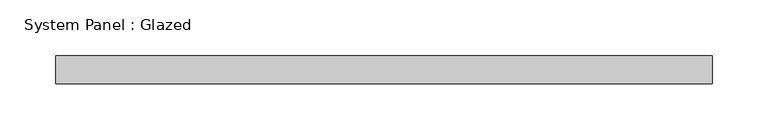
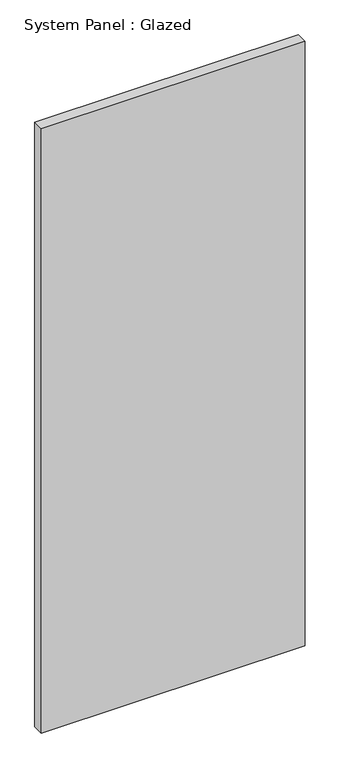
"""IFC4 building model written with IfcOpenShell, lengths in millimetres: plate geometry, System Panel : Glazed."""

from ifc_helpers import new_model, si_unit, origin, origin_with_axes, place, context, project, spatial, polyline, outline, extrude, source, transform, mapped, element, save


def system_panel_glazed_c088aa0a(model_context):
    return source(origin(), model_context, "Body", "SweptSolid", [
        extrude(outline(polyline([(295.275, 19.05), (-295.275, 19.05), (-295.275, 44.45), (295.275, 44.45), (295.275, 19.05)])), origin_with_axes(), (0.0, 0.0, 1.0), 1430.3709712),
    ])


if __name__ == "__main__":
    model = new_model("IFC4")
    model_context = context("Model", 3, world=origin())
    ifc_project = project(units=[si_unit("LENGTHUNIT", "METRE", prefix="MILLI")], contexts=[model_context])
    site = spatial("IfcSite", under=ifc_project)
    building = spatial("IfcBuilding", under=site)
    placement = place(None, origin())
    system_panel_glazed_shape = system_panel_glazed_c088aa0a(model_context)
    element("IfcPlate", 1, ObjectType="System Panel : Glazed", at=placement, inside=building, context=model_context, shape_type="MappedRepresentation", body=[
        mapped(system_panel_glazed_shape, transform((0.0, 0.0, 0.0), x_axis=(1.0, 0.0, 0.0), y_axis=(0.0, 1.0, 0.0), z_axis=(0.0, 0.0, 1.0))),
    ])
    save(model, "model.ifc")

# Revit data of these elements
# Type "System Panel : Glazed"
#   Construction Type Id = "GSP4R"
#   Analytic Construction = "1/8 in Pilkington single glazing"
#   Visual Light Transmittance = 0.9
#   Solar Heat Gain Coefficient = 0.86
#   Heat Transfer Coefficient (U) = 1.18115 BTU/(h·ft²·°F)
#   Define Thermal Properties by = 1
# Element 1 (IfcPlate, "System Panel : Glazed")
#   Materials on its faces: "Glass"
# Materials
#   "Glass": class "Glass", colour RGB 0 128 192, transparency 0.75, Description = "Soda Lime Glass", Cost = 0
